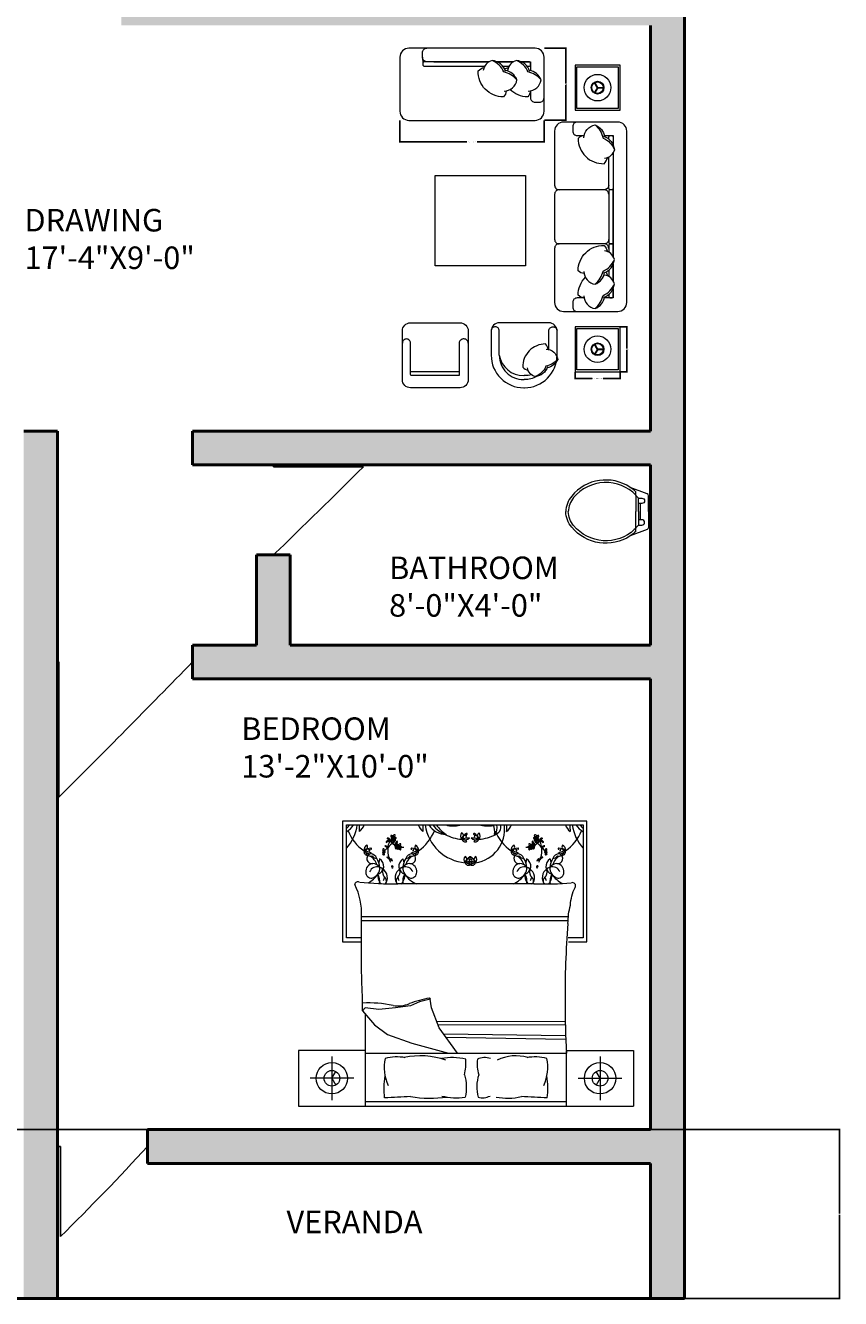
# Model space of a CAD drawing. Units: inches. Extents: x -17 to 536, y -817 to 53.
# Tile 3 of 9: x 319 to 536, y -775 to -436. Entities that reach past the tile are written whole.
import ezdxf

# ---------------------------------------------------------------- set-up
doc = ezdxf.new("R2010")
doc.units = ezdxf.units.IN
doc.header["$MEASUREMENT"] = 0
for name, color, linetype, lineweight in [('A-ANNO-DIMS', 2, 'Continuous', 18), ('A-AREA-IDEN', 7, 'Continuous', 18), ('A-DOOR', 4, 'Continuous', 25), ('A-FLOR-FIXT', 9, 'Continuous', 18), ('A-FURN', 8, 'Continuous', 13), ('A-WALL', 7, 'Continuous', 50), ('A-WALL-PATT', 22, 'Continuous', 13)]:
    doc.layers.add(name, color=color, linetype=linetype, lineweight=lineweight)
doc.styles.get("Standard").update_dxf_attribs({"font": 'arial.ttf'})
doc.dimstyles.get("Standard").update_dxf_attribs({"dimtxt": 0.18, "dimasz": 0.18, "dimexe": 0.18, "dimexo": 0.0625, "dimgap": 0.09, "dimtad": 0, "dimtih": 1, "dimtoh": 1, "dimdec": 0, "dimzin": 0, "dimdsep": 46, "dimlunit": 3, "dimtxsty": 'Standard', "dimcen": 0.09, "dimadec": 0, "dimazin": 0, "dimtfac": 1, "dimtdec": 0, "dimtofl": 0, "dimtmove": 0, "dimatfit": 3, "dimfxl": 1, "dimtolj": 1, "dimtzin": 0, "dimarcsym": 0})

# ---------------------------------------------------------------- blocks, each defined once
blk = doc.blocks.new('DAY BED1')
at = {"color": 0}
blk.add_line((0.3, 0.25), (0.225, 0.255), dxfattribs=at)
blk.add_lwpolyline([(-0.3, 0, -0.414214), (-0.4, 0.1), (-0.4, 0.1, 0.317837), (-0.4, 0.1, -0.414214), (-0.4, 0.1), (-0.4, 0.1, 1.186185), (-0.4, 0.1, -0.414214), (-0.4, 0.1), (-0.4, 1.5, -0.414214), (-0.3, 1.6), (0.3, 1.6, -0.414214), (0.4, 1.5), (0.4, 0.1, -0.414214), (0.3, 0)], format="xyb", close=True, dxfattribs=at)
for points in [[(-0.073, 1.45), (-0.15, 1.45, -0.414214), (-0.2, 1.5), (-0.2, 1.55, -0.414214), (-0.15, 1.6)], [(-0.076, 1.425, -0.356772), (0.05, 1.568, -0.249542), (0.154, 1.438, 9.61688)], [(0.05, 1.568, -0.14773), (0.136, 1.422, -0.213343), (0.262, 1.293, -0.178662)], [(-0.073, 1.45, 0.165541), (-0.139, 1.419, 0.200231), (-0.058, 1.221, 0.121523)], [(0.143, 1.442, -0.306663), (0.262, 1.293, -0.30633), (0.154, 1.196, 0.872847)], [(0.25, 1.345), (0.25, 1.45), (0.152, 1.45, -0.414214)], [(0.2, 1.412), (0.2, 1.43, -0.414214), (0.22, 1.45), (0.23, 1.45, -0.414214), (0.25, 1.43)], [(0.25, 1.43), (0.25, 1.345, -0.414214)], [(-0.076, 1.156, -0.356772), (0.05, 1.299, -0.249542), (0.154, 1.169, 9.61688)], [(0.05, 1.299, -0.14773), (0.136, 1.153, -0.213343), (0.262, 1.024, -0.178662)], [(-0.073, 1.181, 0.165541), (-0.139, 1.15, 0.425989), (0.148, 0.869, 0.121523), (0.187, 0.936, -7.115464)], [(0.143, 1.173, -0.306663), (0.262, 1.024, -0.30633), (0.154, 0.926, 0.872847)], [(0.168, 1.163, 0.071865), (0.187, 1.205, -7.115464)], [(0.2, 1.142), (0.2, 1.211, -0.414214)], [(0.25, 1.262), (0.25, 1.075, -0.414214)], [(0.25, 0.992), (0.25, 0.275, -0.414214), (0.23, 0.255), (0.22, 0.255, -0.414214), (0.2, 0.275), (0.2, 0.942, -0.414214)], [(0.25, 0.377), (0.25, 0.3, 0.414214), (0.3, 0.25), (0.35, 0.25, 0.414214), (0.4, 0.3)]]:
    blk.add_lwpolyline(points, format="xyb", dxfattribs=at)
for points in [[(0.25, 1.075), (0.25, 1.262)], [(0.25, 0.377), (0.25, 0.992)]]:
    blk.add_lwpolyline(points, dxfattribs=at)
blk = doc.blocks.new('BED-WITH-NIGHTSTANDS-STANDARD')
for p, q in [((11.79, 75.95), (11.79, 43.78)), ((76.89, 75.95), (11.79, 75.95)), ((12.82, 74.91), (75.86, 74.91)), ((12.82, 44.81), (12.82, 74.91)), ((75.86, 74.91), (75.86, 44.81)), ((76.89, 43.78), (76.89, 75.95)), ((21.62, 65.86), (21.42, 64.85)), ((27.86, 65.86), (28.06, 64.85)), ((60.82, 65.86), (60.62, 64.85)), ((67.06, 65.86), (67.25, 64.85)), ((62.78, 59.23), (26.52, 59.23)), ((71.93, 50.46), (16.83, 50.46)), ((71.85, 49.35), (16.83, 49.35)), ((16.84, 44.81), (12.82, 44.81)), ((75.86, 44.81), (71.92, 44.81)), ((11.79, 43.78), (16.84, 43.78)), ((71.94, 43.78), (76.89, 43.78)), ((32.25, 27.79), (29.9, 26.71)), ((35.15, 28.52), (32.25, 27.79)), ((35.51, 26.17), (35.15, 28.52)), ((17.78, 26.17), (17.06, 25.44)), ((17.06, 25.44), (20.32, 21.65)), ((21.4, 25.8), (17.78, 26.17)), ((17.86, 0), (17.86, 24.51)), ((25.92, 26.17), (21.4, 25.8)), ((29.9, 26.71), (25.92, 26.17)), ((37.5, 20.92), (35.51, 26.17)), ((20.32, 21.65), (23.75, 19.12)), ((71.13, 22.47), (36.86, 22.61)), ((71.12, 21.55), (37.21, 21.69)), ((42.39, 14.11), (37.5, 20.92)), ((23.75, 19.12), (30.26, 16.77)), ((71.17, 18.74), (38.74, 19.2)), ((71.2, 17.82), (39.41, 18.27)), ((17.86, 14.11), (71.44, 14.11)), ((30.26, 16.77), (40, 14.11)), ((8.93, 13.28), (8.93, 1.61)), ((80.37, 13.28), (80.37, 1.61)), ((14.76, 7.44), (3.1, 7.44)), ((74.54, 7.44), (86.21, 7.44)), ((0, 0), (89.3, 0)), ((71.44, 1.15), (17.86, 1.15))]:
    blk.add_line(p, q)
for points in [[(16.87, 33.62, -0.001242), (16.83, 50.56, 0.127202), (15.04, 59.01)], [(71.82, 48.64, -0.056112), (72.47, 53.56, -0.095341), (73.73, 58.29)], [(22.99, 2.23, -0.074897), (23.1, 8.06, 0.472817)], [(44.23, 8.39, -0.14099), (44.41, 2.43, -0.235245)], [(48.05, 8.39, 0.14099), (47.87, 2.43, 0.235245)], [(66.31, 2.23, 0.074897), (66.2, 8.06, -0.472817)]]:
    blk.add_lwpolyline(points, format="xyb")
for points in [[(17.86, 14.88), (0, 14.88), (0, 0)], [(71.44, 0), (71.44, 14.88), (89.3, 14.88), (89.3, 0)], [(8.93, 7.44), (9.97, 9.25)], [(8.93, 7.44), (9.97, 5.64)], [(80.37, 7.44), (79.33, 9.25)], [(80.37, 7.44), (79.33, 5.64)]]:
    blk.add_lwpolyline(points)
for centre, radius in [((25.29, 71.49), 0.227), ((63.39, 71.49), 0.227), ((26.78, 69.09), 0.227), ((61.9, 69.09), 0.227), ((8.93, 7.44), 4.17), ((80.37, 7.44), 4.17), ((8.93, 7.44), 2.08), ((80.37, 7.44), 2.08)]:
    blk.add_circle(centre, radius)
for centre, radius, start, end in [((7.95, 79.1), 7.08, 313.5186, 323.6964), ((9.99, 78.04), 5.68, 299.8884, 326.5383), ((4.14, 76.48), 11.66, 318.1144, 352.255), ((13.17, 76.73), 4.74, 311.0454, 337.4453), ((0.19, 74.18), 16.13, 356.3481, 2.5919), ((36.31, 76.73), 4.74, 202.5547, 228.9546), ((49.3, 74.18), 16.13, 177.4081, 183.6519), ((45.35, 76.48), 11.66, 187.745, 265.5377), ((39.5, 78.04), 5.68, 213.4617, 268.728), ((41.54, 79.1), 7.08, 216.3036, 252.1496), ((45.26, 81.09), 10.53, 215.947, 235.9877), ((41.19, 81.04), 6.41, 252.9798, 286.4569), ((43.73, 84.35), 9.48, 264.3643, 265.6213), ((48.73, 90.84), 16.94, 250.0972, 250.2783), ((45.93, 73.79), 9.03, 278.1803, 7.1364), ((50.46, 81.04), 6.41, 253.5431, 287.0202), ((47.92, 84.35), 9.48, 274.3787, 275.6357), ((42.93, 90.84), 16.94, 289.7217, 289.9028), ((47.1, 72.96), 5.22, 353.3805, 21.883), ((51.89, 74.42), 2.09, 280.9261, 13.6102), ((50.32, 74.13), 2.65, 318.0951, 17.1391), ((39.38, 74.18), 16.13, 356.3481, 2.5919), ((52.37, 76.73), 4.74, 311.0454, 337.4453), ((75.51, 76.73), 4.74, 202.5547, 228.9546), ((88.49, 74.18), 16.13, 177.4081, 183.6519), ((84.54, 76.48), 11.66, 187.745, 221.8856), ((78.69, 78.04), 5.68, 213.4617, 240.1116), ((80.73, 79.1), 7.08, 216.3036, 226.4814), ((24.09, 77.63), 11.66, 201.4092, 235.6135), ((23.83, 71.16), 0.254, 55.6077, 145.6462), ((23.65, 70.61), 0.687, 21.7087, 93.0299), ((20.03, 65.71), 6.64, 53.6254, 57.3216), ((23.86, 70.79), 0.592, 342.8042, 79.6943), ((24.82, 71.92), 0.225, 134.3732, 211.9501), ((25.23, 72.18), 0.717, 211.9501, 255.2442), ((24.83, 71.66), 0.449, 8.5614, 112.5914), ((25.04, 71.17), 0.31, 88.5719, 233.8954), ((24.96, 71.68), 0.151, 352.868, 97.094), ((24.8, 71.35), 0.313, 298.8493, 359.9355), ((24.87, 71.09), 0.358, 4.2123, 48.1587), ((25.6, 71.91), 0.375, 100.9597, 208.7804), ((25.56, 71.27), 0.217, 178.1325, 268.8919), ((26.01, 71.41), 0.69, 132.3896, 156.5724), ((25.71, 71.32), 0.372, 42.3208, 130.2111), ((25.79, 71.71), 0.47, 226.3462, 279.6513), ((25.29, 72.11), 0.529, 291.6382, 4.947), ((25.3, 70.84), 0.547, 7.4968, 71.2737), ((25.7, 72.2), 0.745, 254.2829, 276.9148), ((25.64, 72.14), 0.174, 4.947, 127.5263), ((25.84, 71.44), 0.196, 279.6513, 42.3208), ((25.39, 77.63), 11.66, 304.3865, 338.5908), ((44.45, 82.73), 11.66, 242.5854, 265.5377), ((44.5, 71.97), 1.29, 140.8855, 222.2127), ((43.03, 71.93), 0.974, 301.6373, 61.4609), ((44.5, 71.14), 0.954, 76.148, 182.2415), ((46.34, 70.15), 2.95, 121.989, 161.0841), ((45.99, 63.32), 8.16, 92.7418, 107.407), ((44.3, 72.78), 1.84, 245.6899, 314.4589), ((44.7, 71.94), 0.126, 140.0755, 76.148), ((44.85, 72.52), 0.145, 288.4408, 121.989), ((44.87, 72.45), 0.0704, 171.9833, 288.4408), ((45.67, 63.32), 8.16, 72.593, 87.2582), ((47.35, 72.78), 1.84, 225.5411, 294.3101), ((46.81, 72.52), 0.145, 58.011, 251.5592), ((46.78, 72.45), 0.0704, 251.5592, 8.0167), ((46.95, 71.89), 0.076, 103.9791, 39.8091), ((45.32, 70.15), 2.95, 18.9159, 58.011), ((47.16, 71.14), 0.954, 357.7585, 103.852), ((48.62, 71.93), 0.974, 118.5391, 238.3627), ((47.15, 71.97), 1.29, 317.7873, 39.1145), ((47.2, 82.73), 11.66, 274.4623, 297.4146), ((63.28, 77.63), 11.66, 201.4092, 235.6135), ((62.84, 71.44), 0.196, 137.6792, 260.3487), ((62.97, 71.32), 0.372, 49.7889, 137.6792), ((62.89, 71.71), 0.47, 260.3487, 313.6538), ((63.38, 70.84), 0.547, 108.7263, 172.5032), ((63.39, 72.11), 0.529, 175.053, 248.3618), ((63.04, 72.14), 0.174, 52.4737, 175.053), ((62.98, 72.2), 0.745, 263.0852, 285.7171), ((63.12, 71.27), 0.217, 271.1081, 1.8675), ((62.67, 71.41), 0.69, 23.4276, 47.6104), ((63.08, 71.91), 0.375, 331.2196, 79.0403), ((63.85, 71.66), 0.449, 67.4086, 171.4386), ((63.81, 71.09), 0.358, 131.8413, 175.7877), ((63.72, 71.68), 0.151, 82.906, 187.132), ((63.88, 71.35), 0.313, 180.0645, 241.1507), ((63.45, 72.18), 0.717, 284.7558, 328.0499), ((63.64, 71.17), 0.31, 306.1046, 91.4281), ((63.86, 71.92), 0.225, 328.0499, 45.6268), ((64.81, 70.79), 0.592, 100.3057, 197.1958), ((65.03, 70.61), 0.687, 86.9701, 158.2913), ((64.85, 71.16), 0.254, 34.3538, 124.3923), ((68.65, 65.71), 6.64, 122.6784, 126.3746), ((64.59, 77.63), 11.66, 304.3865, 338.5908), ((18.77, 68.29), 1.29, 110.9613, 192.2885), ((18.44, 67.78), 0.967, 166.272, 267.0484), ((17.48, 68.98), 0.974, 271.7131, 31.5367), ((19.45, 65.79), 2.95, 92.0648, 131.1598), ((18.35, 67.57), 0.954, 46.2238, 152.3173), ((15.74, 60.05), 8.16, 62.8176, 77.4827), ((19, 69.09), 1.84, 215.7657, 284.5347), ((16.47, 66.31), 1.99, 14.7031, 58.6173), ((18.92, 68.17), 0.126, 110.2817, 46.2238), ((19.33, 68.52), 0.0704, 142.0591, 258.5166), ((19.35, 68.59), 0.145, 258.5166, 92.0648), ((22.68, 68.16), 0.375, 100.9597, 142.2379), ((22.37, 67.74), 0.227, 273.2768, 86.7232), ((23.09, 67.66), 0.69, 132.3896, 156.5724), ((22.78, 67.57), 0.372, 42.3208, 130.2111), ((22.36, 68.36), 0.529, 291.6382, 4.947), ((22.72, 68.39), 0.174, 4.947, 127.5263), ((17.62, 74.63), 8.48, 307.9541, 316.8459), ((22.91, 67.69), 0.196, 279.6513, 42.3208), ((23.13, 66.79), 2.52, 82.8698, 91.6736), ((23.48, 69.5), 0.469, 205.5379, 258.6744), ((22.81, 67.91), 1.41, 59.344, 79.7412), ((23.64, 70.33), 0.254, 123.0979, 213.1364), ((22.5, 67.92), 1.43, 43.6929, 51.7899), ((24.07, 69.96), 0.687, 92.3172, 160.5201), ((27.22, 64.73), 6.64, 121.1156, 124.8118), ((23.38, 68.86), 0.429, 355.7131, 81.6568), ((24, 70.22), 0.592, 82.6008, 147.1845), ((23.14, 68.48), 0.748, 27.3659, 59.344), ((23.71, 68.98), 0.182, 202.5583, 304.2343), ((23.92, 70.2), 0.263, 45.7354, 121.1156), ((31.19, 68.33), 7.4, 176.1723, 196.4158), ((27.5, 68.52), 3.71, 150.7959, 175.244), ((32.84, 60.63), 12.2, 127.8256, 137.7588), ((23.81, 70.85), 0.263, 338.2452, 53.6254), ((24.24, 70.68), 0.198, 158.2452, 340.6395), ((24.24, 70.53), 0.198, 225.7354, 48.1297), ((27.97, 72.33), 3.96, 201.7087, 206.2181), ((24.82, 69.63), 1.04, 40.9365, 112.7695), ((24.48, 69.98), 0.61, 49.3812, 95.5456), ((27.5, 68.52), 3.71, 137.5083, 145.9967), ((24.92, 70.22), 0.63, 61.1838, 141.6792), ((27.89, 73.45), 4.45, 220.182, 239.456), ((25.01, 71.09), 0.223, 228.2946, 6.2474), ((25.35, 71), 0.733, 229.3812, 289.9959), ((25.61, 71.14), 0.379, 183.635, 258.4363), ((24.88, 70.1), 0.753, 15.6484, 62.2957), ((25.68, 70.87), 0.176, 215.0752, 14.7644), ((25.31, 70.6), 1.04, 287.889, 359.722), ((25.28, 70.11), 0.61, 305.1128, 351.2773), ((25.59, 68.99), 0.63, 3.8774, 87.1501), ((25.15, 69.23), 0.61, 352.0748, 38.2393), ((25.04, 68.75), 1.04, 343.6301, 55.4631), ((26.48, 69.05), 0.733, 172.0748, 232.6895), ((25.77, 70.21), 0.63, 271.4625, 339.4747), ((26.61, 69.9), 0.733, 110.6625, 171.2773), ((25.47, 68.96), 0.753, 318.342, 4.9894), ((26.3, 69.52), 0.225, 134.3732, 211.9501), ((27.89, 73.45), 4.45, 246.1523, 246.9499), ((26.72, 69.78), 0.717, 211.9501, 255.2442), ((26.32, 69.27), 0.449, 8.5614, 112.5914), ((26.53, 68.78), 0.31, 88.5719, 233.8954), ((25.66, 70.27), 0.753, 338.3627, 25.0101), ((26.5, 68.69), 0.223, 228.2946, 6.2474), ((26.44, 69.28), 0.151, 352.868, 97.094), ((26.29, 68.96), 0.313, 298.8493, 359.9355), ((26.36, 68.69), 0.358, 4.2123, 48.1587), ((27.09, 69.51), 0.375, 100.9597, 208.7804), ((27.1, 68.74), 0.379, 183.635, 258.4363), ((27.05, 68.88), 0.217, 178.1325, 268.8919), ((27.5, 69.01), 0.69, 132.3896, 156.5724), ((27.19, 68.93), 0.372, 42.3208, 130.2111), ((27.28, 69.31), 0.47, 226.3462, 279.6513), ((26.77, 69.71), 0.529, 291.6382, 4.947), ((26.79, 68.44), 0.547, 7.4968, 71.2737), ((27.19, 69.8), 0.745, 254.2829, 276.9148), ((27.13, 69.74), 0.174, 4.947, 127.5263), ((27.16, 68.47), 0.176, 215.0752, 14.7644), ((27.32, 69.04), 0.196, 279.6513, 42.3208), ((27.89, 73.45), 4.45, 265.2415, 272.8929), ((30.14, 68.59), 0.145, 87.9352, 281.4834), ((30.48, 69.09), 1.84, 255.4653, 324.2343), ((33.75, 60.05), 8.16, 102.5173, 117.1824), ((30.04, 65.79), 2.95, 48.8402, 87.9352), ((30.16, 68.52), 0.0704, 281.4834, 37.9409), ((31.14, 67.57), 0.954, 27.6827, 133.7762), ((30.58, 68.12), 0.076, 133.7729, 69.7333), ((32.01, 68.98), 0.974, 148.4633, 268.2869), ((31.04, 67.78), 0.967, 272.9516, 13.728), ((33.02, 66.31), 1.99, 121.3827, 165.2969), ((30.72, 68.29), 1.29, 347.7115, 69.0387), ((43.49, 69.11), 1.99, 44.6273, 88.5415), ((44.47, 71.37), 0.967, 196.1963, 296.9726), ((48.16, 69.11), 1.99, 91.4585, 135.3727), ((47.18, 71.37), 0.967, 243.0274, 343.8037), ((57.96, 68.29), 1.29, 110.9613, 192.2885), ((57.64, 67.78), 0.967, 166.272, 267.0484), ((56.67, 68.98), 0.974, 271.7131, 31.5367), ((58.64, 65.79), 2.95, 92.0648, 131.1598), ((57.54, 67.57), 0.954, 46.2238, 152.3173), ((55.66, 66.31), 1.99, 14.7031, 58.6173), ((58.19, 69.09), 1.84, 215.7657, 284.5347), ((54.93, 60.05), 8.16, 62.8176, 77.4827), ((58.12, 68.17), 0.126, 110.2817, 46.2238), ((58.52, 68.52), 0.0704, 142.0591, 258.5166), ((58.54, 68.59), 0.145, 258.5166, 92.0648), ((60.79, 73.45), 4.45, 267.1071, 274.7585), ((61.36, 69.04), 0.196, 137.6792, 260.3487), ((61.49, 68.93), 0.372, 49.7889, 137.6792), ((61.4, 69.31), 0.47, 260.3487, 313.6538), ((61.52, 68.47), 0.176, 165.2356, 324.9248), ((61.89, 68.44), 0.547, 108.7263, 172.5032), ((61.55, 69.74), 0.174, 52.4737, 175.053), ((61.91, 69.71), 0.529, 175.053, 248.3618), ((61.49, 69.8), 0.745, 263.0852, 285.7171), ((61.63, 68.88), 0.217, 271.1081, 1.8675), ((61.18, 69.01), 0.69, 23.4276, 47.6104), ((61.59, 69.51), 0.375, 331.2196, 79.0403), ((61.58, 68.74), 0.379, 281.5637, 356.365), ((62.36, 69.27), 0.449, 67.4086, 171.4386), ((62.32, 68.69), 0.358, 131.8413, 175.7877), ((62.18, 68.69), 0.223, 173.7526, 311.7054), ((62.23, 69.28), 0.151, 82.906, 187.132), ((62.39, 68.96), 0.313, 180.0645, 241.1507), ((61.96, 69.78), 0.717, 284.7558, 328.0499), ((62.15, 68.78), 0.31, 306.1046, 91.4281), ((63.02, 70.27), 0.753, 154.9899, 201.6373), ((62.91, 70.21), 0.63, 200.5253, 268.5375), ((63.37, 70.6), 1.04, 180.278, 252.111), ((62.07, 69.9), 0.733, 8.7227, 69.3375), ((63.21, 68.96), 0.753, 175.0106, 221.658), ((63.08, 68.99), 0.63, 92.8499, 176.1226), ((62.38, 69.52), 0.225, 328.0499, 45.6268), ((60.79, 73.45), 4.45, 293.0501, 293.8477), ((63.64, 68.75), 1.04, 124.5369, 196.3699), ((62.2, 69.05), 0.733, 307.3105, 7.9252), ((63.4, 70.11), 0.61, 188.7227, 234.8872), ((63, 70.87), 0.176, 165.2356, 324.9248), ((63.53, 69.23), 0.61, 141.7607, 187.9252), ((60.79, 73.45), 4.45, 300.544, 319.818), ((63.8, 70.1), 0.753, 117.7043, 164.3516), ((63.86, 69.63), 1.04, 67.2305, 139.0635), ((63.33, 71), 0.733, 250.0041, 310.6188), ((63.07, 71.14), 0.379, 281.5637, 356.365), ((55.84, 60.63), 12.2, 42.2412, 52.1744), ((63.67, 71.09), 0.223, 173.7526, 311.7054), ((63.75, 70.22), 0.63, 38.3208, 118.8162), ((64.2, 69.98), 0.61, 84.4544, 130.6188), ((61.17, 68.52), 3.71, 34.0033, 42.4917), ((64.44, 70.53), 0.198, 131.8703, 314.2646), ((64.44, 70.68), 0.198, 199.3605, 21.7548), ((60.71, 72.33), 3.96, 333.7819, 338.2913), ((61.17, 68.52), 3.71, 4.756, 29.2041), ((64.76, 70.2), 0.263, 58.8844, 134.2646), ((57.49, 68.33), 7.4, 343.5842, 3.8277), ((64.86, 70.85), 0.263, 126.3746, 201.7548), ((64.68, 70.22), 0.592, 32.8155, 97.3992), ((64.6, 69.96), 0.687, 19.4799, 87.6828), ((65.3, 68.86), 0.429, 98.3432, 184.2869), ((65.53, 68.48), 0.748, 120.656, 152.6341), ((64.97, 68.98), 0.182, 235.7657, 337.4417), ((71.06, 74.63), 8.48, 223.1541, 232.0459), ((61.46, 64.73), 6.64, 55.1882, 58.8844), ((66.18, 67.92), 1.43, 128.2101, 136.3071), ((65.87, 67.91), 1.41, 100.2588, 120.656), ((65.04, 70.33), 0.254, 326.8636, 56.9021), ((65.55, 66.79), 2.52, 88.3264, 97.1302), ((65.2, 69.5), 0.469, 281.3256, 334.4621), ((65.76, 67.69), 0.196, 137.6792, 260.3487), ((65.89, 67.57), 0.372, 49.7889, 137.6792), ((65.96, 68.39), 0.174, 52.4737, 175.053), ((66.31, 68.36), 0.529, 175.053, 248.3618), ((65.59, 67.66), 0.69, 23.4276, 47.6104), ((66, 68.16), 0.375, 37.7621, 79.0403), ((66.31, 67.74), 0.227, 93.2768, 266.7232), ((69.33, 68.59), 0.145, 87.9352, 281.4834), ((72.94, 60.05), 8.16, 102.5173, 117.1824), ((69.68, 69.09), 1.84, 255.4653, 324.2343), ((69.23, 65.79), 2.95, 48.8402, 87.9352), ((69.35, 68.52), 0.0704, 281.4834, 37.9409), ((70.33, 67.57), 0.954, 27.6827, 133.7762), ((69.77, 68.12), 0.076, 133.7729, 69.7333), ((71.2, 68.98), 0.974, 148.4633, 268.2869), ((72.21, 66.31), 1.99, 121.3827, 165.2969), ((70.23, 67.78), 0.967, 272.9516, 13.728), ((69.91, 68.29), 1.29, 347.7115, 69.0387), ((20.07, 62.49), 2.13, 97.1143, 185.0551), ((19.58, 65.93), 1.34, 109.1312, 279.736), ((19.3, 67.38), 0.821, 216.7319, 296.0245), ((16.92, 62.98), 4.22, 18.2955, 58.7386), ((19.26, 65.53), 1.67, 15.6955, 94.031), ((21.06, 67.75), 1.78, 218.4175, 263.8338), ((19.7, 62.02), 2.59, 35.9599, 87.6409), ((16.88, 63.32), 4.79, 3.4924, 33.7117), ((20.52, 63.93), 2.22, 286.8663, 60.0915), ((22.69, 67.39), 0.379, 217.3642, 258.4363), ((22.64, 67.53), 0.217, 178.1325, 268.8919), ((22.87, 67.96), 0.47, 226.3462, 279.6513), ((22.38, 67.09), 0.547, 7.4968, 71.2737), ((22.78, 68.45), 0.745, 254.2829, 276.9148), ((22.75, 67.12), 0.176, 215.0752, 14.7644), ((23.66, 63.78), 2.52, 82.8698, 91.6736), ((24.01, 66.5), 0.469, 205.5379, 258.6744), ((23.34, 64.91), 1.41, 59.344, 79.7412), ((23.03, 64.91), 1.43, 43.6929, 51.7899), ((23.91, 65.86), 0.429, 355.7131, 81.6568), ((23.68, 65.48), 0.748, 27.3659, 59.344), ((24.24, 65.97), 0.182, 202.5583, 304.2343), ((31.19, 68.33), 7.4, 200.1059, 206.9968), ((24.57, 65.46), 0.429, 36.5232, 122.4668), ((24.35, 65.08), 0.748, 58.836, 90.8141), ((24.52, 65.8), 0.182, 173.9457, 275.6216), ((24.16, 64.24), 1.43, 66.3901, 74.4871), ((25.09, 65.85), 0.469, 219.5056, 272.6421), ((24.01, 64.51), 1.41, 38.4388, 58.836), ((22.86, 64.26), 2.52, 26.5064, 35.3102), ((28.97, 63.93), 2.22, 119.9085, 253.1337), ((29.79, 62.02), 2.59, 92.3591, 144.0401), ((32.6, 63.32), 4.79, 146.2883, 176.5076), ((32.56, 62.98), 4.22, 121.2614, 161.7045), ((30.23, 65.53), 1.67, 85.969, 164.3045), ((28.42, 67.75), 1.78, 276.1662, 321.5825), ((29.91, 65.93), 1.34, 260.264, 70.8688), ((29.42, 62.49), 2.13, 354.9449, 82.8857), ((30.18, 67.38), 0.821, 243.9755, 323.2681), ((45.4, 65.72), 1.29, 140.8855, 222.2127), ((43.93, 65.68), 0.974, 301.6373, 61.4609), ((47.23, 63.9), 2.95, 121.989, 161.0841), ((45.39, 64.89), 0.954, 76.148, 182.2415), ((45.2, 66.54), 1.84, 245.6899, 314.4589), ((46.88, 57.07), 8.16, 92.7418, 107.407), ((45.37, 65.13), 0.967, 196.1963, 296.9726), ((44.39, 62.86), 1.99, 44.6273, 88.5415), ((46.46, 66.54), 1.84, 225.5411, 294.3101), ((44.78, 57.07), 8.16, 72.593, 87.2582), ((45.59, 65.7), 0.126, 140.0755, 76.148), ((45.74, 66.28), 0.145, 288.4408, 121.989), ((45.77, 66.21), 0.0704, 171.9833, 288.4408), ((45.91, 66.28), 0.145, 58.011, 251.5592), ((46.29, 65.13), 0.967, 243.0274, 343.8037), ((47.27, 62.86), 1.99, 91.4585, 135.3727), ((45.89, 66.21), 0.0704, 251.5592, 8.0167), ((46.05, 65.65), 0.076, 103.9791, 39.8091), ((44.43, 63.9), 2.95, 18.9159, 58.011), ((46.26, 64.89), 0.954, 357.7585, 103.852), ((47.73, 65.68), 0.974, 118.5391, 238.3627), ((46.26, 65.72), 1.29, 317.7873, 39.1145), ((59.26, 62.49), 2.13, 97.1143, 185.0551), ((58.77, 65.93), 1.34, 109.1312, 279.736), ((58.5, 67.38), 0.821, 216.7319, 296.0245), ((56.12, 62.98), 4.22, 18.2955, 58.7386), ((58.45, 65.53), 1.67, 15.6955, 94.031), ((60.25, 67.75), 1.78, 218.4175, 263.8338), ((58.89, 62.02), 2.59, 35.9599, 87.6409), ((56.08, 63.32), 4.79, 3.4924, 33.7117), ((59.71, 63.93), 2.22, 286.8663, 60.0915), ((64.67, 64.51), 1.41, 121.164, 141.5612), ((65.82, 64.26), 2.52, 144.6898, 153.4936), ((63.59, 65.85), 0.469, 267.3579, 320.4944), ((64.11, 65.46), 0.429, 57.5332, 143.4768), ((64.33, 65.08), 0.748, 89.1859, 121.164), ((64.52, 64.24), 1.43, 105.5129, 113.6099), ((57.49, 68.33), 7.4, 333.0032, 339.8941), ((64.16, 65.8), 0.182, 264.3784, 6.0543), ((64.77, 65.86), 0.429, 98.3432, 184.2869), ((65, 65.48), 0.748, 120.656, 152.6341), ((64.44, 65.97), 0.182, 235.7657, 337.4417), ((65.65, 64.91), 1.43, 128.2101, 136.3071), ((65.34, 64.91), 1.41, 100.2588, 120.656), ((65.02, 63.78), 2.52, 88.3264, 97.1302), ((64.67, 66.5), 0.469, 281.3256, 334.4621), ((65.81, 67.96), 0.47, 260.3487, 313.6538), ((66.3, 67.09), 0.547, 108.7263, 172.5032), ((65.92, 67.12), 0.176, 165.2356, 324.9248), ((65.9, 68.45), 0.745, 263.0852, 285.7171), ((68.16, 63.93), 2.22, 119.9085, 253.1337), ((66.04, 67.53), 0.217, 271.1081, 1.8675), ((65.99, 67.39), 0.379, 281.5637, 322.6358), ((68.98, 62.02), 2.59, 92.3591, 144.0401), ((71.8, 63.32), 4.79, 146.2883, 176.5076), ((71.76, 62.98), 4.22, 121.2614, 161.7045), ((69.42, 65.53), 1.67, 85.969, 164.3045), ((67.62, 67.75), 1.78, 276.1662, 321.5825), ((69.1, 65.93), 1.34, 260.264, 70.8688), ((68.61, 62.49), 2.13, 354.9449, 82.8857), ((69.38, 67.38), 0.821, 243.9755, 323.2681), ((19.45, 62.27), 1.51, 178.9462, 275.5144), ((15.52, 65.52), 6.76, 296.7003, 326.3329), ((20.91, 61.68), 2.07, 68.5779, 158.4181), ((18.99, 63.39), 2.69, 283.079, 4.7067), ((24.57, 61.5), 3.44, 175.2696, 214.215), ((17.99, 59.89), 3.7, 350.8446, 31.1782), ((24.57, 61.5), 3.44, 143.6555, 147.2989), ((21.92, 63), 0.554, 344.8529, 102.6959), ((20.86, 60.85), 2.85, 330.8249, 70.7178), ((24.22, 62.38), 1.83, 164.8529, 228.4347), ((20.43, 61.37), 2.57, 330.0851, 352.564), ((25, 63.84), 0.172, 79.5616, 257.2949), ((24.98, 63.73), 0.28, 259.5864, 79.5616), ((28.63, 60.85), 2.85, 109.2822, 209.1751), ((25.26, 62.38), 1.83, 311.5653, 15.1471), ((29.06, 61.37), 2.57, 187.436, 209.9149), ((27.56, 63), 0.554, 77.3041, 195.1471), ((24.91, 61.5), 3.44, 32.7011, 36.3445), ((24.91, 61.5), 3.44, 325.785, 4.7304), ((31.49, 59.89), 3.7, 148.8218, 190.2867), ((30.5, 63.39), 2.69, 175.2933, 256.921), ((28.58, 61.68), 2.07, 21.5819, 111.4221), ((33.97, 65.52), 6.76, 213.6671, 248.5059), ((30.03, 62.27), 1.51, 264.4856, 1.0538), ((58.65, 62.27), 1.51, 178.9462, 275.5144), ((54.71, 65.52), 6.76, 291.4941, 326.3329), ((60.1, 61.68), 2.07, 68.5779, 158.4181), ((58.18, 63.39), 2.69, 283.079, 4.7067), ((63.77, 61.5), 3.44, 175.2696, 214.215), ((57.19, 59.89), 3.7, 349.7133, 31.1782), ((63.77, 61.5), 3.44, 143.6555, 147.2989), ((61.11, 63), 0.554, 344.8529, 102.6959), ((60.05, 60.85), 2.85, 330.8249, 70.7178), ((63.42, 62.38), 1.83, 164.8529, 228.4347), ((59.62, 61.37), 2.57, 330.0851, 352.564), ((63.7, 63.73), 0.28, 100.4384, 280.4136), ((63.68, 63.84), 0.172, 282.7051, 100.4384), ((67.82, 60.85), 2.85, 109.2822, 209.1751), ((64.46, 62.38), 1.83, 311.5653, 15.1471), ((68.25, 61.37), 2.57, 187.436, 209.9149), ((66.76, 63), 0.554, 77.3041, 195.1471), ((64.11, 61.5), 3.44, 32.7011, 36.3445), ((64.11, 61.5), 3.44, 325.785, 4.7304), ((70.68, 59.89), 3.7, 148.8218, 190.751), ((69.69, 63.39), 2.69, 175.2933, 256.921), ((67.77, 61.68), 2.07, 21.5819, 111.4221), ((73.16, 65.52), 6.76, 213.6671, 246.3547), ((69.23, 62.27), 1.51, 264.4856, 1.0538), ((15.86, 58.95), 0.824, 62.6588, 176.02), ((25.46, 152.19), 92.96, 264.3113, 270.6567), ((22.58, 60.22), 1.08, 217.675, 239.9707), ((22.12, 60.01), 1.34, 336.1646, 48.4347), ((22.58, 60.22), 1.08, 296.442, 315.5483), ((27.36, 60.01), 1.34, 131.5653, 203.8354), ((26.91, 60.22), 1.08, 224.4517, 246.771), ((26.91, 60.22), 1.08, 293.2856, 322.325), ((61.77, 60.22), 1.08, 217.675, 246.7144), ((61.77, 60.22), 1.08, 293.2856, 315.5483), ((61.32, 60.01), 1.34, 336.1646, 48.4347), ((65.51, 146.09), 86.9, 268.1965, 274.7598), ((66.56, 60.01), 1.34, 131.5653, 203.8354), ((66.1, 60.22), 1.08, 224.4517, 253.3657), ((66.1, 60.22), 1.08, 287.4186, 322.325), ((73.05, 58.74), 0.814, 326.1736, 113.4781), ((280.38, 30.86), 209.31, 175.1265, 180.8855), ((-64.82, 27.66), 81.91, 358.447, 4.1706), ((18.59, -6.18), 33.7, 78.6608, 92.5481), ((26.65, 33.99), 7.27, 258.6608, 293.7384), ((41.35, -5.23), 34.63, 100.6617, 109.8806), ((34.95, 28.59), 0.215, 340.2464, 91.1377), ((231.53, 25.03), 160.46, 179.0718, 183.9), ((34.37, 10.4), 11.51, 168.2417, 204.8684), ((26.18, 1.18), 11.97, 78.9631, 104.8961), ((32.48, -7.33), 20.76, 70.7385, 101.9603), ((40.88, -2.79), 15.75, 76.3762, 100.1383), ((33.71, 11.37), 10.94, 344.1707, 5.9871), ((58.57, 11.37), 10.94, 174.0129, 195.8293), ((49.69, 8.22), 4.73, 71.4593, 114.9817), ((57.96, 2.06), 11.37, 73.8254, 116.1239), ((63.13, 1.18), 11.97, 75.1039, 101.0369), ((54.94, 10.4), 11.51, 335.1316, 11.7583), ((72.21, -847.63), 851.28, 92.85022, 93.31479), ((35.23, 34.54), 32.39, 260.503, 277.7804), ((42.07, 18.17), 15.91, 256.04, 278.4751), ((49.09, 6.68), 4.42, 253.8974, 296.6563), ((55.71, 17.85), 15.7, 258.8159, 283.6573), ((17.09, -847.63), 851.28, 86.68521, 87.14978)]:
    blk.add_arc(centre, radius, start, end)
blk = doc.blocks.new('WC-22IN')
for p, q in [((18.71, 12.76), (18.71, 13.68)), ((18.71, 12.76), (18.71, 8.42)), ((18.71, 4.08), (18.71, 8.42)), ((18.71, 3.16), (18.71, 4.08))]:
    blk.add_line(p, q)
for points in [[(17.19, 14.88, 0.383919), (1.59, 12.57, 0.163732), (0, 8.42, 0.359733)], [(18.71, 12.76, 0.448546), (2.1, 12.15, 0.162618), (0.66, 8.42, 0.470877)], [(18.71, 13.68, 0.040937), (17.19, 14.88, 0.163732)], [(22.05, 8.42), (22.05, 12.63, 0.31031), (21.69, 13.15), (17.19, 14.88, 0.209071)], [(19.37, 12, 0.022712), (18.71, 12.76, 0.162618)], [(19.37, 8.42), (19.37, 12, 0.476108)], [(19.37, 12), (20.3, 12, -1), (20.3, 10.59), (19.82, 10.59)], [(17.19, 1.97, -0.383919), (1.59, 4.28, -0.163732), (0, 8.42, -0.359733)], [(18.26, 3.64, -0.431639), (2.1, 4.7, -0.162618), (0.66, 8.42, -0.470877)], [(22.05, 8.42), (22.05, 4.21, -0.31031), (21.69, 3.7), (17.19, 1.97, -0.209071)], [(19.37, 8.42), (19.37, 4.85, -0.022712)], [(18.71, 4.08, -0.014165), (18.26, 3.64, -0.162618)], [(19.37, 4.85, -0.022712), (18.71, 4.08, -0.162618)], [(19.37, 4.85), (20.3, 4.85, 1), (20.3, 6.25), (19.82, 6.25)], [(18.71, 3.16, -0.040937), (17.19, 1.97, -0.163732)]]:
    blk.add_lwpolyline(points, format="xyb")
for points in [[(19.82, 10.59), (19.37, 10.59)], [(19.82, 10.59), (19.82, 6.25)], [(19.82, 6.25), (19.37, 6.25)]]:
    blk.add_lwpolyline(points)
blk = doc.blocks.new('END-TABLE-LAMP-B')
for p, q in [((5.94, 5.97), (5.09, 7.43)), ((6.07, 6.04), (5.22, 7.51)), ((5.94, 6.04), (5.09, 4.58)), ((6.07, 5.97), (5.22, 4.5)), ((6, 6.08), (7.7, 6.08)), ((6, 5.93), (7.7, 5.93))]:
    blk.add_line(p, q)
at = {"ltscale": 0.03}
blk.add_lwpolyline([(0, 12.01), (0, 0), (12.01, 0), (12.01, 12.01)], close=True, dxfattribs=at)
blk.add_lwpolyline([(0.48, 0.48), (0.48, 11.53), (11.53, 11.53), (11.53, 0.48)], close=True)
for radius in [3.54, 1.7, 1.52]:
    blk.add_circle((6, 6), radius)
blk = doc.blocks.new('*D26')
at = {"layer": 'A-ANNO-DIMS', "color": 0, "lineweight": -2, "transparency": 16777216}
for p, q in [((418.57, -461.78), (418.57, -467.66)), ((457, -461.78), (457, -467.66)), ((418.75, -467.48), (436.39, -467.48)), ((456.82, -467.48), (439.18, -467.48))]:
    blk.add_line(p, q, dxfattribs=at)
at = {"layer": 'A-ANNO-DIMS', "color": 0, "transparency": 16777216}
for points in [[(418.75, -467.45), (418.75, -467.51), (418.57, -467.48)], [(456.82, -467.45), (456.82, -467.51), (457, -467.48)]]:
    blk.add_solid(points, dxfattribs=at)
at = {"layer": 'Defpoints', "color": 0, "transparency": 16777216}
for p in [(418.57, -461.71), (457, -461.71), (457, -467.48)]:
    blk.add_point(p, dxfattribs=at)
at = {"layer": 'A-ANNO-DIMS', "color": 0, "transparency": 16777216, "insert": (437.79, -467.48), "char_height": 0.18, "attachment_point": 5}
blk.add_mtext('\\A1;DAYBED 3\'-2 1/2" TYP.', dxfattribs=at)
blk = doc.blocks.new('*D27')
at = {"layer": 'A-ANNO-DIMS', "color": 0, "lineweight": -2, "transparency": 16777216}
for p, q in [((457.07, -442.5), (462.95, -442.5)), ((462.77, -442.68), (462.77, -451.93)), ((462.77, -461.53), (462.77, -452.29)), ((457.07, -461.71), (462.95, -461.71))]:
    blk.add_line(p, q, dxfattribs=at)
at = {"layer": 'A-ANNO-DIMS', "color": 0, "transparency": 16777216}
for points in [[(462.74, -442.68), (462.8, -442.68), (462.77, -442.5)], [(462.74, -461.53), (462.8, -461.53), (462.77, -461.71)]]:
    blk.add_solid(points, dxfattribs=at)
at = {"layer": 'Defpoints', "color": 0, "transparency": 16777216}
for p in [(457, -442.5), (462.77, -442.5), (457, -461.71)]:
    blk.add_point(p, dxfattribs=at)
at = {"layer": 'A-ANNO-DIMS', "color": 0, "transparency": 16777216, "insert": (462.77, -452.11), "char_height": 0.18, "attachment_point": 5}
blk.add_mtext('\\A1;1\'-7" TYP.', dxfattribs=at)
blk = doc.blocks.new('*D34')
at = {"layer": 'A-ANNO-DIMS', "color": 0, "lineweight": -2, "transparency": 16777216}
for p, q in [((465.25, -528.73), (465.25, -530.65)), ((477.26, -528.73), (477.26, -530.65)), ((465.43, -530.47), (469.77, -530.47)), ((477.08, -530.47), (472.74, -530.47))]:
    blk.add_line(p, q, dxfattribs=at)
at = {"layer": 'A-ANNO-DIMS', "color": 0, "transparency": 16777216}
for points in [[(465.43, -530.44), (465.43, -530.5), (465.25, -530.47)], [(477.08, -530.44), (477.08, -530.5), (477.26, -530.47)]]:
    blk.add_solid(points, dxfattribs=at)
at = {"layer": 'Defpoints', "color": 0, "transparency": 16777216}
for p in [(465.25, -528.67), (477.26, -528.67), (477.26, -530.47)]:
    blk.add_point(p, dxfattribs=at)
at = {"layer": 'A-ANNO-DIMS', "color": 0, "transparency": 16777216, "insert": (471.25, -530.47), "char_height": 0.18, "attachment_point": 5}
blk.add_mtext('\\A1;END TABLE B 1\'-0" TYP.', dxfattribs=at)
blk = doc.blocks.new('*D35')
at = {"layer": 'A-ANNO-DIMS', "color": 0, "lineweight": -2, "transparency": 16777216}
for p, q in [((477.32, -516.66), (479.24, -516.66)), ((479.06, -516.84), (479.06, -522.48)), ((479.06, -528.49), (479.06, -522.85)), ((477.32, -528.67), (479.24, -528.67))]:
    blk.add_line(p, q, dxfattribs=at)
at = {"layer": 'A-ANNO-DIMS', "color": 0, "transparency": 16777216}
for points in [[(479.03, -516.84), (479.09, -516.84), (479.06, -516.66)], [(479.03, -528.49), (479.09, -528.49), (479.06, -528.67)]]:
    blk.add_solid(points, dxfattribs=at)
at = {"layer": 'Defpoints', "color": 0, "transparency": 16777216}
for p in [(477.26, -516.66), (479.06, -516.66), (477.26, -528.67)]:
    blk.add_point(p, dxfattribs=at)
at = {"layer": 'A-ANNO-DIMS', "color": 0, "transparency": 16777216, "insert": (479.06, -522.67), "char_height": 0.18, "attachment_point": 5}
blk.add_mtext('\\A1;1\'-0" TYP.', dxfattribs=at)
blk = doc.blocks.new('*D39')
at = {"layer": 'A-ANNO-DIMS', "color": 0, "lineweight": -2, "transparency": 16777216}
for p, q in [((217.43, -730.45), (535.9, -730.45)), ((535.72, -730.63), (535.72, -752.77)), ((535.72, -775.27), (535.72, -753.13)), ((217.43, -775.45), (535.9, -775.45))]:
    blk.add_line(p, q, dxfattribs=at)
at = {"layer": 'A-ANNO-DIMS', "color": 0, "transparency": 16777216}
for points in [[(535.69, -730.63), (535.75, -730.63), (535.72, -730.45)], [(535.69, -775.27), (535.75, -775.27), (535.72, -775.45)]]:
    blk.add_solid(points, dxfattribs=at)
at = {"layer": 'Defpoints', "color": 0, "transparency": 16777216}
for p in [(217.37, -730.45), (217.37, -775.45), (535.72, -775.45)]:
    blk.add_point(p, dxfattribs=at)
at = {"layer": 'A-ANNO-DIMS', "color": 0, "transparency": 16777216, "insert": (535.72, -752.95), "char_height": 0.18, "attachment_point": 5}
blk.add_mtext('\\A1;3\'-9"', dxfattribs=at)

msp = doc.modelspace()

# ---------------------------------------------------------------- hatches: boundary and pattern name
at = {"layer": 'A-WALL-PATT'}
h = msp.add_hatch(color=256, dxfattribs=at)
h.dxf.hatch_style = 1
h.paths.add_polyline_path([(217.37, -544.45), (208.37, -544.45), (208.37, -775.45), (217.37, -775.45)], flags=17)
h.paths.add_polyline_path([(327.37, -544.45), (318.37, -544.45), (318.37, -775.45), (327.37, -775.45)], flags=17)
h.paths.add_polyline_path([(494.37, 11.55), (41.37, 11.55), (41.37, -775.45), (50.37, -775.45), (50.37, -739.45), (184.37, -739.45), (184.37, -730.45), (50.37, -730.45), (50.37, -610.45), (172.37, -610.45), (172.37, -601.45), (155.37, -601.45), (155.37, -577.45), (146.37, -577.45), (146.37, -601.45), (50.37, -601.45), (50.37, -553.45), (172.37, -553.45), (172.37, -544.45), (50.37, -544.45), (50.37, -436.45), (191.37, -436.45), (191.37, -319.45), (182.37, -319.45), (182.37, -427.45), (50.37, -427.45), (50.37, -283.45), (98.37, -283.45), (98.37, -274.45), (50.37, -274.45), (50.37, -219.45), (122.37, -219.45), (122.37, -283.45), (191.37, -283.45), (191.37, -274.45), (131.37, -274.45), (131.37, -219.45), (131.37, -150.45), (146.37, -150.45), (146.37, -141.45), (122.37, -141.45), (122.37, -210.45), (50.37, -210.45), (50.37, -150.45), (98.37, -150.45), (98.37, -141.45), (50.37, -141.45), (50.37, 2.55), (182.37, 2.55), (182.37, -150.45), (191.37, -150.45), (191.37, 2.55), (263.37, 2.55), (263.37, -141.45), (227.37, -141.45), (227.37, -150.45), (263.37, -150.45), (263.37, -553.45), (272.37, -553.45), (272.37, -150.45), (308.37, -150.45), (308.37, -141.45), (272.37, -141.45), (272.37, 2.55), (344.37, 2.55), (344.37, -150.45), (353.37, -150.45), (353.37, 2.55), (485.37, 2.55), (485.37, -141.45), (437.37, -141.45), (437.37, -150.45), (485.37, -150.45), (485.37, -210.45), (413.37, -210.45), (413.37, -141.45), (389.37, -141.45), (389.37, -150.45), (404.37, -150.45), (404.37, -219.45), (404.37, -274.45), (353.37, -274.45), (344.37, -274.45), (344.37, -283.45), (353.37, -283.45), (413.37, -283.45), (413.37, -219.45), (485.37, -219.45), (485.37, -274.45), (437.37, -274.45), (437.37, -283.45), (485.37, -283.45), (485.37, -427.45), (353.37, -427.45), (353.37, -319.45), (344.37, -319.45), (344.37, -436.45), (485.37, -436.45), (485.37, -544.45), (363.37, -544.45), (363.37, -553.45), (485.37, -553.45), (485.37, -601.45), (389.37, -601.45), (389.37, -577.45), (380.37, -577.45), (380.37, -601.45), (363.37, -601.45), (363.37, -610.45), (485.37, -610.45), (485.37, -730.45), (351.37, -730.45), (351.37, -739.45), (485.37, -739.45), (485.37, -775.45), (494.37, -775.45)])

# ---------------------------------------------------------------- linework, layer by layer
at = {"layer": 'A-DOOR'}
for p, q in [((384.87, -553.96), (384.87, -553.45)), ((384.87, -553.96), (408.87, -553.96)), ((327.72, -605.95), (327.37, -605.95)), ((327.72, -605.95), (327.72, -641.95)), ((328.16, -734.95), (327.37, -734.95)), ((328.16, -734.95), (328.16, -758.95))]:
    msp.add_line(p, q, dxfattribs=at)
for centre, radius, start, end in [((-1008.54, 869.85), 2009.05, 313.91307, 314.87094), ((-2463.25, 2157.42), 3952.97, 314.91388, 315.64822), ((-148.32, -275.01), 679.14, 314.55501, 317.37177)]:
    msp.add_arc(centre, radius, start, end, dxfattribs=at)
at = {"layer": 'A-FURN', "ltscale": 0.03}
for points in [[(462.21, -462.17, 0.414214), (459.81, -464.57), (459.81, -478.98, 0.414214), (461.01, -480.18, 0.414214), (459.81, -481.39), (459.81, -493.4, 0.414214), (461.01, -494.6, 0.414214), (459.81, -495.8), (459.81, -510.21, 0.414214), (462.21, -512.61), (476.63, -512.61, 0.414214), (479.03, -510.21), (479.03, -464.57, 0.414214), (476.63, -462.17)], [(421.41, -532.93), (421.41, -532.93, -0.414214), (419.24, -530.77), (419.24, -517.77, -0.414214), (421.41, -515.61), (421.41, -515.61), (434.62, -515.61, -0.414214), (436.78, -517.77), (436.78, -530.77, -0.414214), (434.62, -532.93)]]:
    msp.add_lwpolyline(points, format="xyb", close=True, dxfattribs=at)
at = {"layer": 'A-FURN'}
for points in [[(465.82, -462.17, 0.414214), (464.62, -463.37), (464.62, -464.57, 0.414214), (465.82, -465.77), (467.68, -465.77)], [(467.6, -466.38, -0.356772), (470.63, -462.93, -0.249542), (473.13, -466.05, 9.61688)], [(470.63, -462.93, -0.14773), (472.7, -466.44, -0.213343), (475.72, -469.54, -0.178662)], [(467.68, -465.77, 0.165541), (466.09, -466.51, 0.425989), (472.97, -473.26, 0.121523), (473.92, -471.66, -7.115464)], [(472.86, -465.96, -0.306663), (475.72, -469.54, -0.30633), (473.11, -471.88, 0.872847)], [(474.22, -466.69), (474.22, -466.25, -0.414214), (474.7, -465.77), (474.94, -465.77, -0.414214), (475.42, -466.25)], [(475.42, -466.25), (475.42, -468.3, -0.414214)], [(475.42, -470.3), (475.42, -479.7, -0.414214), (474.94, -480.18), (474.7, -480.18, -0.414214), (474.22, -479.7), (474.22, -471.51, -0.414214)], [(474.22, -478.98, -0.414214), (473.02, -480.18), (461.01, -480.18, -0.414214)], [(474.22, -481.39, 0.414214), (473.02, -480.18)], [(474.22, -495.8, 0.414214), (473.02, -494.6), (461.01, -494.6, 0.414214)], [(474.22, -493.4, -0.414214), (473.02, -494.6)], [(475.42, -498.01), (475.42, -495.08, 0.414214), (474.94, -494.6), (474.7, -494.6, 0.414214), (474.22, -495.08), (474.22, -496.8, 0.414214)], [(467.68, -502.54, -0.165541), (466.09, -501.8, -0.425989), (472.97, -495.05, -0.121523), (473.92, -496.65, 7.115464)], [(472.86, -502.35, 0.306663), (475.72, -498.77, 0.30633), (473.11, -496.43, -0.872847)], [(470.63, -505.38, 0.14773), (472.7, -501.87, 0.213343), (475.72, -498.77, 0.178662)], [(474.22, -501.62), (474.22, -503.27, 0.414214)], [(475.42, -504.48), (475.42, -500.01, 0.414214)], [(467.68, -509.01, -0.165541), (466.09, -508.27, -0.200231), (468.02, -503.5, -0.121523)], [(467.6, -501.94, 0.356772), (470.63, -505.38, 0.249542), (473.13, -502.26, -9.61688)], [(472.86, -508.82, 0.306663), (475.72, -505.24, 0.30633), (473.11, -502.9, -0.872847)], [(473.45, -502.12, -0.071865), (473.92, -503.12, 7.115464)], [(467.6, -508.41, 0.356772), (470.63, -511.85, 0.249542), (473.13, -508.73, -9.61688)], [(470.63, -511.85, 0.14773), (472.7, -508.34, 0.213343), (475.72, -505.24, 0.178662)], [(475.42, -506.48), (475.42, -509.01), (473.06, -509.01, 0.414214)], [(474.22, -508.09), (474.22, -508.53, 0.414214), (474.7, -509.01), (474.94, -509.01, 0.414214), (475.42, -508.53)], [(475.42, -508.53), (475.42, -506.48, 0.414214)], [(467.68, -509.01), (465.82, -509.01, 0.414214), (464.62, -510.21), (464.62, -511.41, 0.414214), (465.82, -512.61)], [(445.07, -524.27), (445.07, -517.77, 0.414214), (443.99, -516.69), (443.99, -516.69, 0.414214), (442.91, -517.77)], [(458.28, -522.75), (458.28, -517.77, -0.414214), (459.37, -516.69), (459.37, -516.69, -0.414214), (460.45, -517.77)], [(421.41, -529.03), (421.41, -521.02, 0.414214), (420.33, -519.94), (420.33, -519.94, 0.414214), (419.24, -521.02)], [(436.78, -521.02, 0.414214), (435.7, -519.94), (435.48, -519.94, 0.414214), (434.4, -521.02), (434.4, -522.7)], [(458.07, -522.7, 0.165541), (457.4, -521.27, 0.425989), (451.32, -527.47, 0.121523), (452.76, -528.33, -7.115464)], [(445.07, -524.27, 0.372719), (451.57, -529.68), (451.68, -529.68)], [(445.07, -524.27, 0.414214), (451.57, -530.77), (451.68, -530.77)], [(460.63, -525.36, -0.14773), (457.46, -527.22, -0.213343), (454.67, -529.95, -0.178662)], [(457.52, -522.63, -0.356772), (460.63, -525.36, -0.249542), (457.81, -527.61, 9.61688)], [(430.32, -529.68), (421.84, -529.68, -0.414214), (421.41, -529.25), (421.41, -529.03, -0.414214), (421.84, -528.6), (429.23, -528.6, -0.414214)], [(429.23, -528.6), (433.97, -528.6, -0.414214), (434.4, -529.03), (434.4, -529.25, -0.414214), (433.97, -529.68)], [(457.9, -527.37, -0.306663), (454.67, -529.95, -0.30633), (452.56, -527.6, 0.872847)], [(433.97, -529.68), (430.32, -529.68, -0.414214)], [(453.63, -529.45, -0.072384), (451.79, -529.68), (451.68, -529.68)], [(455.01, -529.91, -0.130591), (451.79, -530.77), (451.68, -530.77)]]:
    msp.add_lwpolyline(points, format="xyb", dxfattribs=at)
for points in [[(473.06, -465.77), (475.42, -465.77), (475.42, -468.3)], [(475.42, -470.3), (475.42, -498.01)], [(475.42, -500.01), (475.42, -504.48)], [(434.4, -522.7), (434.4, -529.68), (430.32, -529.68)], [(430.32, -529.68), (421.52, -529.68)]]:
    msp.add_lwpolyline(points, dxfattribs=at)
at = {"layer": 'A-FURN', "ltscale": 0.03}
msp.add_lwpolyline([(428.02, -500.45), (428.02, -476.43), (452.04, -476.43), (452.04, -500.45)], close=True, dxfattribs=at)
at = {"layer": 'A-FURN'}
msp.add_lwpolyline([(475.42, -494.12), (475.42, -480.66, 0.414214), (474.94, -480.18), (474.7, -480.18, 0.414214), (474.22, -480.66), (474.22, -494.12, 0.414214), (474.7, -494.6), (474.94, -494.6, 0.414214)], format="xyb", close=True, dxfattribs=at)
at = {"layer": 'A-FURN', "ltscale": 0.03}
msp.add_lwpolyline([(451.68, -515.61), (445.07, -515.61, 0.414214), (442.91, -517.77), (442.91, -524.27, 0.414214), (451.57, -532.93), (451.68, -532.93), (451.79, -532.93, 0.414214), (460.45, -524.27), (460.45, -517.77, 0.414214), (458.28, -515.61), (451.68, -515.61)], format="xyb", dxfattribs=at)
at = {"layer": 'A-WALL'}
for p, q in [((494.37, 11.55), (494.37, -775.45)), ((485.37, -436.45), (485.37, -544.45)), ((318.37, -544.45), (327.37, -544.45)), ((327.37, -544.45), (327.37, -775.45)), ((363.37, -553.45), (363.37, -544.45)), ((363.37, -544.45), (485.37, -544.45)), ((363.37, -553.45), (485.37, -553.45)), ((485.37, -553.45), (485.37, -601.45)), ((380.37, -577.45), (380.37, -601.45)), ((380.37, -577.45), (389.37, -577.45)), ((389.37, -577.45), (389.37, -601.45)), ((363.37, -601.45), (380.37, -601.45)), ((363.37, -601.45), (363.37, -610.45)), ((389.37, -601.45), (485.37, -601.45)), ((363.37, -610.45), (485.37, -610.45)), ((485.37, -610.45), (485.37, -730.45)), ((351.37, -730.45), (485.37, -730.45)), ((351.37, -739.45), (351.37, -730.45)), ((351.37, -739.45), (485.37, -739.45)), ((485.37, -739.45), (485.37, -775.45)), ((41.37, -775.45), (353.37, -775.45)), ((353.37, -775.45), (494.37, -775.45))]:
    msp.add_line(p, q, dxfattribs=at)

# ---------------------------------------------------------------- block references
at = {"layer": 'A-FLOR-FIXT'}
msp.add_blockref('WC-22IN', (462.78, -574.33), dxfattribs=at)
at = {"layer": 'A-FURN', "ltscale": 0.03, "xscale": -24.01965723609237, "yscale": 24.01965723609237, "zscale": 24.01965723609237, "rotation": 270}
msp.add_blockref('DAY BED1', (418.57, -452.11), dxfattribs=at)
at = {"layer": 'A-FURN'}
for name, p in [('END-TABLE-LAMP-B', (465.25, -459.01)), ('END-TABLE-LAMP-B', (465.25, -528.67)), ('BED-WITH-NIGHTSTANDS-STANDARD', (391.54, -724.25))]:
    msp.add_blockref(name, p, dxfattribs=at)

# ---------------------------------------------------------------- texts
at = {"layer": 'A-AREA-IDEN', "char_height": 6, "attachment_point": 1}
for s, insert in [('DRAWING\\P17\'-4"X9\'-0"', (318.57, -485.31)), ('BATHROOM\\P8\'-0"X4\'-0"', (415.71, -577.88)), ('BEDROOM\\P13\'-2"X10\'-0"', (376.33, -620.71)), ('VERANDA', (388.38, -752.05))]:
    msp.add_mtext(s, dxfattribs=dict(at, insert=insert))

# ---------------------------------------------------------------- dimensions: what is measured, and where the dimension line sits
at = {"layer": 'A-ANNO-DIMS'}
for base, p1, p2, picture, middle in [((462.77, -442.5), (457, -461.71), (457, -442.5), '*D27', (462.77, -452.11)), ((479.06, -516.66), (477.26, -528.67), (477.26, -516.66), '*D35', (479.06, -522.67))]:
    dim = msp.add_linear_dim(base=base, p1=p1, p2=p2, angle=90, text='<> TYP.', dimstyle='Standard', override={"dimdec": 1, "dimlfac": 1, "dimrnd": 0, "dimzin": 1, "dimdsep": 46, "dimlunit": 4, "dimfrac": 2}, dxfattribs=at)
    dim.commit()
    dim.dimension.update_dxf_attribs({"geometry": picture, "text_midpoint": middle})
for base, p1, p2, text, picture, middle in [((457, -467.48), (418.57, -461.71), (457, -461.71), 'DAYBED <> TYP.', '*D26', (437.79, -467.48)), ((477.26, -530.47), (465.25, -528.67), (477.26, -528.67), 'END TABLE B <> TYP.', '*D34', (471.25, -530.47))]:
    dim = msp.add_linear_dim(base=base, p1=p1, p2=p2, text=text, dimstyle='Standard', override={"dimdec": 1, "dimlfac": 1, "dimrnd": 0, "dimzin": 1, "dimdsep": 46, "dimlunit": 4, "dimfrac": 2}, dxfattribs=at)
    dim.commit()
    dim.dimension.update_dxf_attribs({"geometry": picture, "text_midpoint": middle})
dim = msp.add_linear_dim(base=(535.72, -775.45), p1=(217.37, -730.45), p2=(217.37, -775.45), angle=90, dimstyle='Standard', override={"dimdec": 1, "dimlfac": 1, "dimrnd": 0, "dimzin": 1, "dimdsep": 46, "dimlunit": 4, "dimfrac": 2}, dxfattribs=at)
dim.commit()
dim.dimension.update_dxf_attribs({"geometry": '*D39', "text_midpoint": (535.72, -752.95)})

doc.saveas('drawing.dxf')
